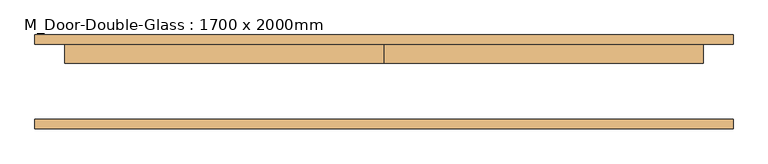
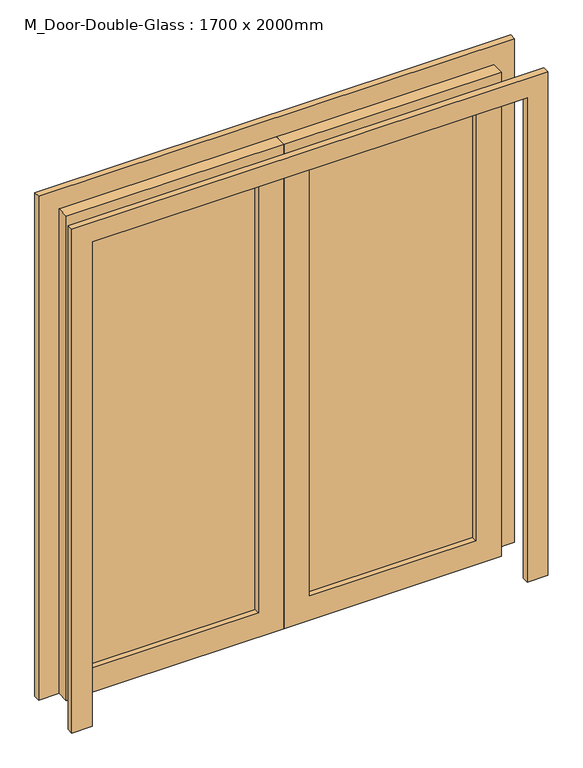
"""IFC4 building model written with IfcOpenShell, lengths in millimetres: door geometry, M_Door-Double-Glass : 1700 x 2000mm."""

from ifc_helpers import new_model, si_unit, frame, origin, place, context, project, spatial, polyline, outline, extrude, source, transform, mapped, element, save


def m_door_double_glass_1700_x_2000mm_d5355b94(model_context):
    return source(origin(), model_context, "Body", "SweptSolid", [
        extrude(outline(polyline([(2000.0, 850.0), (2000.0, 0.0), (0.0, 0.0), (0.0, 850.0), (2000.0, 850.0)]), holes=[polyline([(1900.0, 750.0), (100.0, 750.0), (100.0, 100.0), (1900.0, 100.0), (1900.0, 750.0)])]), frame((0.0, 52.38125, 0.0), z_axis=(0.0, 1.0, 0.0), x_axis=(0.0, 0.0, 1.0)), (0.0, 0.0, 1.0), 50.0),
        extrude(outline(polyline([(2000.0, -850.0), (0.0, -850.0), (0.0, 0.0), (2000.0, 0.0), (2000.0, -850.0)]), holes=[polyline([(1900.0, -750.0), (1900.0, -100.0), (100.0, -100.0), (100.0, -750.0), (1900.0, -750.0)])]), frame((0.0, 52.38125, 0.0), z_axis=(0.0, 1.0, 0.0), x_axis=(0.0, 0.0, 1.0)), (0.0, 0.0, 1.0), 50.0),
        extrude(outline(polyline([(-750.0, 80.55625), (-100.0, 80.55625), (-100.0, 74.20625), (-750.0, 74.20625), (-750.0, 80.55625)])), frame((0.0, 0.0, 100.0), z_axis=(0.0, 0.0, 1.0), x_axis=(1.0, 0.0, 0.0)), (0.0, 0.0, 1.0), 1800.0),
        extrude(outline(polyline([(100.0, 80.55625), (750.0, 80.55625), (750.0, 74.20625), (100.0, 74.20625), (100.0, 80.55625)])), frame((0.0, 0.0, 100.0), z_axis=(0.0, 0.0, 1.0), x_axis=(1.0, 0.0, 0.0)), (0.0, 0.0, 1.0), 1800.0),
        extrude(outline(polyline([(0.0, 930.0), (2080.0, 930.0), (2080.0, -930.0), (0.0, -930.0), (0.0, -850.0), (2000.0, -850.0), (2000.0, 850.0), (0.0, 850.0), (0.0, 930.0)])), frame((0.0, -122.61875, 0.0), z_axis=(0.0, 1.0, 0.0), x_axis=(0.0, 0.0, 1.0)), (0.0, 0.0, 1.0), 25.0),
        extrude(outline(polyline([(0.0, 930.0), (2080.0, 930.0), (2080.0, -930.0), (0.0, -930.0), (0.0, -850.0), (2000.0, -850.0), (2000.0, 850.0), (0.0, 850.0), (0.0, 930.0)])), frame((0.0, 102.38125, 0.0), z_axis=(0.0, 1.0, 0.0), x_axis=(0.0, 0.0, 1.0)), (0.0, 0.0, 1.0), 25.0),
    ])


if __name__ == "__main__":
    model = new_model("IFC4")
    model_context = context("Model", 3, world=origin())
    ifc_project = project(units=[si_unit("LENGTHUNIT", "METRE", prefix="MILLI")], contexts=[model_context])
    site = spatial("IfcSite", under=ifc_project)
    building = spatial("IfcBuilding", under=site)
    placement = place(None, origin())
    m_door_double_glass_1700_x_2000mm_shape = m_door_double_glass_1700_x_2000mm_d5355b94(model_context)
    element("IfcDoor", 1, ObjectType="M_Door-Double-Glass : 1700 x 2000mm", at=placement, inside=building, context=model_context, shape_type="MappedRepresentation", body=[
        mapped(m_door_double_glass_1700_x_2000mm_shape, transform((0.0, 0.0, 0.0), x_axis=(1.0, 0.0, 0.0), y_axis=(0.0, 1.0, 0.0), z_axis=(0.0, 0.0, 1.0))),
    ])
    save(model, "model.ifc")

# Revit data of these elements
# Type "M_Door-Double-Glass : 1700 x 2000mm"
#   Type Mark = "40"
#   Construction Type Id = "opn-d45"
#   Assembly Code = "C1020"
#   Analytic Construction = "Wood frame, double glass door "
#   W = 850 mm
#   Thickness = 50 mm
#   Thermal Resistance (R) = 0.31964 (m²·K)/W
#   Swing Angle [instance default] = 90.00°
#   Heat Transfer Coefficient (U) = 3.12872 W/(m²·K)
#   Height = 2000 mm
#   Bottom Rail = 100 mm
#   Top Rail = 100 mm
#   Stiles = 100 mm
#   Trim Projection = 25 mm
#   Trim Width = 80 mm
#   Width = 1700 mm
#   Define Thermal Properties by = 1
#   Glazing = Glass
#   Panel Material = Wood - Birch - Solid Stained Light Low Gloss
#   Trim Material = Paint - Sienna
#   Visual Light Transmittance = 0
#   Solar Heat Gain Coefficient = 0
#   Function = (empty or 0)
#   Wall Closure = (empty or 0)
# Element 1 (IfcDoor, "M_Door-Double-Glass : 1700 x 2000mm")
#   Materials on its faces: "Wood - Birch - Solid Stained Light Low Gloss", "Paint - Sienna", "Glass"
# Materials
#   "Glass": class "Glass", colour RGB 0 128 192, transparency 0.9, Description = "Soda Lime Glass", Cost = 0
#   "Wood - Birch - Solid Stained Light Low Gloss": class "Wood", colour RGB 210 159 95, transparency 0, Cost = 0
#   "Paint - Sienna": colour RGB 118 70 51, transparency 0, Cost = 0
